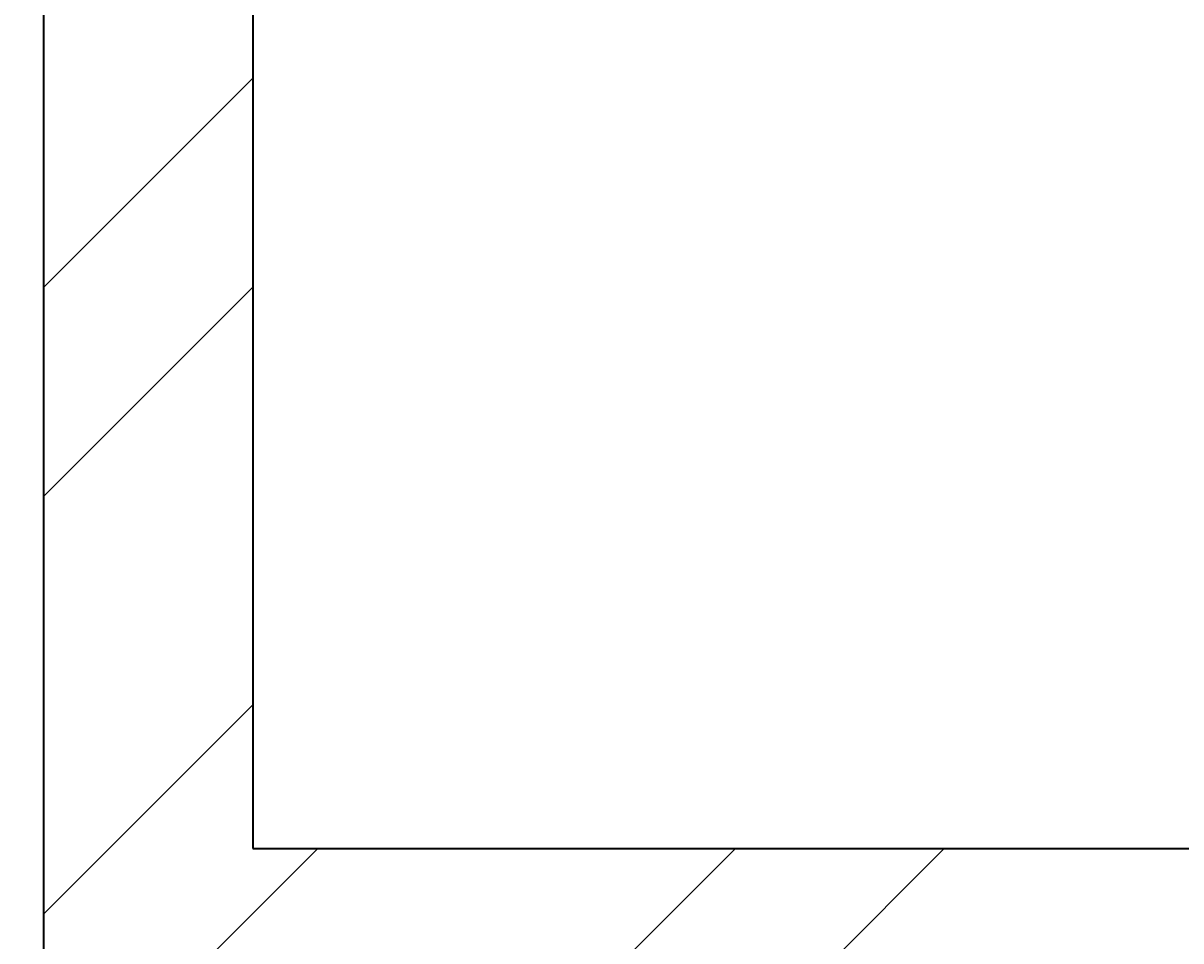
# Model space of a CAD drawing. Units: inches. Extents: x 1885 to 2748, y 783 to 2421.
# Tile 71 of 117: x 1992 to 2017, y 2073 to 2093. Entities that reach past the tile are written whole.
import ezdxf

# ---------------------------------------------------------------- set-up
doc = ezdxf.new("R2010")
doc.units = ezdxf.units.IN
doc.layers.add('A-ANNO-DIMS', color=2, linetype='Continuous', lineweight=18)
doc.layers.add('A-WALL', color=7, linetype='Continuous', lineweight=35)
doc.layers.add('A-WALL-PATT', color=85, linetype='Continuous', lineweight=13, true_color=0x58ba48)
doc.styles.get("Standard").update_dxf_attribs({"font": 'arial.ttf'})
doc.dimstyles.get("Standard").update_dxf_attribs({"dimtxt": 0.18, "dimasz": 0.18, "dimexe": 0.18, "dimexo": 0.0625, "dimgap": 0.09, "dimtad": 0, "dimtih": 1, "dimtoh": 1, "dimdec": 4, "dimzin": 0, "dimdsep": 46, "dimtxsty": 'Standard', "dimcen": 0.09, "dimadec": 0, "dimazin": 0, "dimtfac": 1, "dimtdec": 4, "dimtofl": 0, "dimtmove": 0, "dimatfit": 3, "dimfxl": 1, "dimtolj": 1, "dimtzin": 0, "dimarcsym": 0})

# ---------------------------------------------------------------- blocks, each defined once
blk = doc.blocks.new('*D48')
at = {"layer": 'A-ANNO-DIMS', "color": 0, "lineweight": -2, "transparency": 16777216}
for p, q in [((1980.711, 2348.006), (1902.844, 2348.006)), ((1903.024, 2347.826), (1903.024, 2114.937)), ((1903.024, 1881.686), (1903.024, 2114.574)), ((2016.711, 1881.506), (1902.844, 1881.506))]:
    blk.add_line(p, q, dxfattribs=at)
at = {"layer": 'A-ANNO-DIMS', "color": 0, "transparency": 16777216}
for points in [[(1902.994, 2347.826), (1903.054, 2347.826), (1903.024, 2348.006)], [(1902.994, 1881.686), (1903.054, 1881.686), (1903.024, 1881.506)]]:
    blk.add_solid(points, dxfattribs=at)
at = {"layer": 'Defpoints', "color": 0, "transparency": 16777216}
for p in [(1903.024, 2348.006), (1980.774, 2348.006), (2016.774, 1881.506)]:
    blk.add_point(p, dxfattribs=at)
at = {"layer": 'A-ANNO-DIMS', "color": 0, "transparency": 16777216, "insert": (1903.024, 2114.756), "char_height": 0.18, "attachment_point": 5}
blk.add_mtext('\\A1;466.5', dxfattribs=at)

msp = doc.modelspace()

# ---------------------------------------------------------------- hatches: boundary and pattern name
at = {"layer": 'A-WALL-PATT'}
h = msp.add_hatch(dxfattribs=at)
h.set_pattern_fill('ANSI32', color=256)
h.paths.add_polyline_path([(2007.772, 2318.006), (1980.774, 2318.006), (1980.774, 2281.215), (1985.274, 2281.215), (1985.274, 2313.506), (2007.772, 2313.506), (2007.772, 2315.756)])
h.paths.add_polyline_path([(2094.324, 2318.006), (2067.772, 2318.006), (2067.772, 2313.506), (2094.324, 2313.506), (2094.324, 2315.756)])
h.paths.add_polyline_path([(2131.367, 2315.756), (2131.367, 2318.006), (2131.189, 2318.006), (2112.609, 2318.006), (2112.609, 2313.506), (2117.274, 2313.506), (2117.274, 2255.201), (2121.774, 2255.201), (2121.774, 2313.506), (2131.367, 2313.506)])
h.paths.add_polyline_path([(2190.512, 2318.006), (2155.367, 2318.006), (2155.367, 2313.506), (2169.774, 2313.506), (2169.774, 2229.506), (2121.774, 2229.506), (2121.774, 2233.451), (2119.524, 2233.451), (2117.274, 2233.451), (2117.274, 2201.101), (2121.774, 2201.101), (2121.774, 2225.006), (2169.774, 2225.006), (2169.774, 2165.006), (2306.274, 2165.006), (2306.274, 2066.006), (2310.774, 2066.006), (2344.274, 2066.006), (2486.274, 2066.006), (2486.274, 1886.006), (2483.02, 1886.006), (2483.02, 1881.506), (2486.274, 1881.506), (2486.274, 1880.678), (2490.774, 1880.678), (2490.774, 2070.506), (2344.274, 2070.506), (2310.774, 2070.506), (2310.774, 2165.006), (2310.774, 2173.636), (2308.524, 2173.636), (2306.274, 2173.636), (2306.274, 2169.506), (2174.274, 2169.506), (2174.274, 2313.506), (2190.512, 2313.506), (2190.512, 2315.756)])
h.paths.add_polyline_path([(1985.274, 2221.215), (1980.774, 2221.215), (1980.774, 2165.006), (1992.774, 2165.006), (1992.774, 2141.927), (1997.274, 2141.927), (1997.274, 2165.006), (2117.274, 2165.006), (2117.274, 2163.126), (2121.774, 2163.126), (2121.774, 2172.734), (2119.524, 2172.734), (2117.274, 2172.734), (2117.274, 2169.506), (1985.274, 2169.506)])
h.paths.add_polyline_path([(1997.274, 2105.927), (1992.774, 2105.927), (1992.774, 2070.506), (2016.774, 2070.506), (2016.774, 2059.123), (2019.024, 2059.123), (2021.274, 2059.123), (2021.274, 2070.506), (2117.274, 2070.506), (2117.274, 2022.506), (2114.423, 2022.506), (2114.423, 2018.006), (2123.627, 2018.006), (2123.627, 2020.256), (2123.627, 2022.506), (2121.774, 2022.506), (2121.774, 2142.587), (2119.524, 2142.587), (2117.274, 2142.587), (2117.274, 2075.006), (1997.274, 2075.006)])
h.paths.add_polyline_path([(2092.029, 2020.256), (2092.029, 2022.506), (2021.274, 2022.506), (2021.274, 2035.123), (2016.774, 2035.123), (2016.774, 2018.006), (2016.774, 1978.784), (2021.274, 1978.784), (2021.274, 2018.006), (2092.029, 2018.006)])
h.paths.add_polyline_path([(2260.938, 2022.506), (2153.105, 2022.506), (2153.105, 2020.256), (2153.105, 2018.006), (2155.274, 2018.006), (2155.274, 1886.006), (2107.629, 1886.006), (2107.629, 1881.506), (2182.911, 1881.506), (2182.911, 1883.756), (2182.911, 1886.006), (2159.774, 1886.006), (2159.774, 2018.006), (2260.938, 2018.006), (2260.938, 2020.256)])
h.paths.add_polyline_path([(2047.629, 1883.756), (2047.629, 1886.006), (2021.274, 1886.006), (2021.274, 1918.784), (2019.024, 1918.784), (2016.774, 1918.784), (2016.774, 1881.506), (2047.629, 1881.506)])
h.paths.add_polyline_path([(2306.361, 1883.756), (2306.361, 1886.006), (2296.274, 1886.006), (2296.274, 1982.006), (2316.535, 1982.006), (2316.535, 1984.256), (2316.535, 1986.506), (2296.274, 1986.506), (2296.274, 2022.506), (2289.276, 2022.506), (2289.276, 2018.006), (2291.774, 2018.006), (2291.774, 1886.006), (2242.911, 1886.006), (2242.911, 1881.506), (2306.361, 1881.506)], flags=17)
h.paths.add_polyline_path([(1985.274, 1843.006), (2021.6, 1843.006), (2021.534, 1845.441), (2021.477, 1847.506), (1980.774, 1847.506), (1980.774, 1809.446), (1985.274, 1809.446)])
h.paths.add_polyline_path([(2131.482, 1845.256), (2131.482, 1847.506), (2081.534, 1847.506), (2081.534, 1843.006), (2117.274, 1843.006), (2117.274, 1784.147), (2119.524, 1784.147), (2121.774, 1784.147), (2121.774, 1843.006), (2131.482, 1843.006)])
h.paths.add_polyline_path([(2203.886, 1847.506), (2155.482, 1847.506), (2155.482, 1843.006), (2169.774, 1843.006), (2169.774, 1759.006), (2121.774, 1759.006), (2121.774, 1761.457), (2117.274, 1761.457), (2117.274, 1730.429), (2121.774, 1730.429), (2121.774, 1754.506), (2177.421, 1754.506), (2177.421, 1756.756), (2177.421, 1759.006), (2174.274, 1759.006), (2174.274, 1843.006), (2203.886, 1843.006)])
h.paths.add_polyline_path([(2335.554, 1845.256), (2335.554, 1847.506), (2239.886, 1847.506), (2239.886, 1843.006), (2306.274, 1843.006), (2306.274, 1759.006), (2199.486, 1759.006), (2199.486, 1754.506), (2310.774, 1754.506), (2310.774, 1843.006), (2335.554, 1843.006)])
h.paths.add_polyline_path([(2348.774, 2022.506), (2344.274, 2022.506), (2344.274, 1986.506), (2341.681, 1986.506), (2341.681, 1982.006), (2344.274, 1982.006), (2344.274, 1886.006), (2330.361, 1886.006), (2330.361, 1881.506), (2361.627, 1881.506), (2361.627, 1883.756), (2361.627, 1886.006), (2348.774, 1886.006)], flags=17)
h.paths.add_polyline_path([(2283.251, 2315.756), (2283.251, 2318.006), (2238.512, 2318.006), (2238.512, 2313.506), (2283.251, 2313.506)], flags=17)
h.paths.add_polyline_path([(2363.274, 2348.006), (2388.677, 2348.006), (2388.677, 2350.256), (2388.677, 2352.506), (2358.774, 2352.506), (2358.774, 2348.006), (2358.774, 2318.006), (2344.481, 2318.006), (2344.481, 2313.506), (2358.774, 2313.506), (2358.774, 2229.506), (2310.774, 2229.506), (2310.774, 2231.952), (2306.274, 2231.952), (2306.274, 2205.611), (2310.774, 2205.611), (2310.774, 2225.006), (2358.774, 2225.006), (2358.774, 2211.506), (2452.329, 2211.506), (2452.329, 2213.756), (2452.329, 2216.006), (2363.274, 2216.006), (2363.274, 2318.006)])
h.paths.add_polyline_path([(2310.774, 2313.506), (2320.481, 2313.506), (2320.481, 2315.756), (2320.481, 2318.006), (2302.728, 2318.006), (2302.728, 2313.506), (2306.274, 2313.506), (2306.274, 2251.076), (2310.774, 2251.076)], flags=17)
h.paths.add_polyline_path([(2490.774, 2352.506), (2486.274, 2352.506), (2448.677, 2352.506), (2448.677, 2348.006), (2486.274, 2348.006), (2486.274, 2318.006), (2486.274, 2216.006), (2481.78, 2216.006), (2481.78, 2211.506), (2486.274, 2211.506), (2486.274, 2165.006), (2493.289, 2165.006), (2493.289, 2167.256), (2493.289, 2169.506), (2490.774, 2169.506), (2490.774, 2313.506), (2494.429, 2313.506), (2494.429, 2318.006), (2490.774, 2318.006)])
h.paths.add_polyline_path([(2534.653, 2318.006), (2515.691, 2318.006), (2515.691, 2313.506), (2534.653, 2313.506), (2534.653, 2315.756)])
h.paths.add_polyline_path([(2618.274, 2318.006), (2594.653, 2318.006), (2594.653, 2313.506), (2613.774, 2313.506), (2613.774, 2281.706), (2618.274, 2281.706)])
h.paths.add_polyline_path([(2618.274, 2221.706), (2613.774, 2221.706), (2613.774, 2169.506), (2554.019, 2169.506), (2554.019, 2165.006), (2613.774, 2165.006), (2613.774, 2152.878), (2618.274, 2152.878)])
h.paths.add_polyline_path([(2618.274, 2128.878), (2616.024, 2128.878), (2613.774, 2128.878), (2613.774, 2117.006), (2529.774, 2117.006), (2529.774, 2165.006), (2532.848, 2165.006), (2532.848, 2169.506), (2522.867, 2169.506), (2522.867, 2165.006), (2525.274, 2165.006), (2525.274, 2117.006), (2525.274, 2112.506), (2525.274, 2108.576), (2529.774, 2108.576), (2529.774, 2112.506), (2613.774, 2112.506), (2613.774, 2080.19), (2618.274, 2080.19)])
h.paths.add_polyline_path([(2618.274, 2044.19), (2616.024, 2044.19), (2613.774, 2044.19), (2613.774, 2015.506), (2529.774, 2015.506), (2529.774, 2088.582), (2527.524, 2088.582), (2525.274, 2088.582), (2525.274, 2011.006), (2613.774, 2011.006), (2613.774, 1956.755), (2618.274, 1956.755)])
h.paths.add_polyline_path([(2618.274, 1881.506), (2618.274, 1896.755), (2613.774, 1896.755), (2613.774, 1881.506), (2613.774, 1847.506), (2592.715, 1847.506), (2592.715, 1843.006), (2613.774, 1843.006), (2613.774, 1765.006), (2613.774, 1760.506), (2609.621, 1760.506), (2609.621, 1756.006), (2613.774, 1756.006), (2613.774, 1660.006), (2608.544, 1660.006), (2608.544, 1655.506), (2613.774, 1655.506), (2613.774, 1508.158), (2618.274, 1508.158)])
h.paths.add_polyline_path([(2565.774, 1843.006), (2568.997, 1843.006), (2568.997, 1847.506), (2490.774, 1847.506), (2490.774, 1849.7), (2488.524, 1849.7), (2486.274, 1849.7), (2486.274, 1847.506), (2477.274, 1847.506), (2477.274, 1838.506), (2477.274, 1821.493), (2486.274, 1821.493), (2486.274, 1838.506), (2561.274, 1838.506), (2561.274, 1765.006), (2486.274, 1765.006), (2486.274, 1786.157), (2477.274, 1786.157), (2477.274, 1765.006), (2477.274, 1756.006), (2486.274, 1756.006), (2565.774, 1756.006), (2585.621, 1756.006), (2585.621, 1758.256), (2585.621, 1760.506), (2565.774, 1760.506), (2565.774, 1765.006)])
h.paths.add_polyline_path([(2486.274, 1651.006), (2561.274, 1651.006), (2561.274, 1567.006), (2486.274, 1567.006), (2486.274, 1591.321), (2477.274, 1591.321), (2477.274, 1567.006), (2477.274, 1558.006), (2477.274, 1555.439), (2481.774, 1555.439), (2481.774, 1558.006), (2568.653, 1558.006), (2568.653, 1560.256), (2568.653, 1562.506), (2565.774, 1562.506), (2565.774, 1655.506), (2584.544, 1655.506), (2584.544, 1657.756), (2584.544, 1660.006), (2565.774, 1660.006), (2486.274, 1660.006), (2477.274, 1660.006), (2477.274, 1651.006), (2477.274, 1632.989), (2486.274, 1632.989)])
h.paths.add_polyline_path([(2449.967, 1883.756), (2449.967, 1886.006), (2421.627, 1886.006), (2421.627, 1881.506), (2449.967, 1881.506)], flags=17)
h.paths.add_polyline_path([(2447.274, 1847.506), (2395.554, 1847.506), (2395.554, 1843.006), (2442.774, 1843.006), (2442.774, 1809.27), (2447.274, 1809.27)])
h.paths.add_polyline_path([(1985.274, 1749.446), (1980.774, 1749.446), (1980.774, 1694.504), (1985.274, 1694.504), (1985.274, 1694.506), (1986.897, 1694.506), (1986.897, 1697.78), (1986.897, 1699.006), (1985.274, 1699.006)])
h.paths.add_polyline_path([(2152.774, 1699.006), (2121.774, 1699.006), (2121.774, 1703.668), (2119.524, 1703.668), (2117.274, 1703.668), (2117.274, 1699.006), (2009.219, 1699.006), (2009.219, 1694.506), (2148.274, 1694.506), (2148.274, 1692.631), (2152.774, 1692.631)])
h.paths.add_polyline_path([(2016.274, 1694.506), (2011.774, 1694.506), (2011.774, 1558.006), (2040.806, 1558.006), (2040.806, 1560.256), (2040.806, 1562.506), (2016.274, 1562.506)])
h.paths.add_polyline_path([(2152.774, 1663.017), (2150.524, 1663.017), (2148.274, 1663.017), (2148.274, 1562.506), (2100.806, 1562.506), (2100.806, 1558.006), (2165.119, 1558.006), (2165.119, 1560.256), (2165.119, 1562.506), (2152.774, 1562.506), (2152.774, 1610.506), (2224.774, 1610.506), (2224.774, 1607.99), (2229.274, 1607.99), (2229.274, 1615.006), (2152.774, 1615.006)])
h.paths.add_polyline_path([(2238.613, 1560.256), (2238.613, 1562.506), (2229.274, 1562.506), (2229.274, 1588.756), (2227.024, 1588.763), (2224.774, 1588.771), (2224.774, 1562.506), (2189.119, 1562.506), (2189.119, 1558.006), (2238.613, 1558.006)])
h.paths.add_polyline_path([(2336.024, 1560.256), (2336.024, 1562.506), (2310.774, 1562.506), (2310.774, 1656.347), (2308.524, 1656.347), (2306.274, 1656.347), (2306.274, 1562.506), (2286.613, 1562.506), (2286.613, 1558.006), (2336.024, 1558.006)])
h.paths.add_polyline_path([(2447.274, 1690.968), (2445.024, 1690.968), (2442.774, 1690.968), (2442.774, 1687.006), (2306.274, 1687.006), (2306.274, 1680.75), (2310.774, 1680.75), (2310.774, 1682.506), (2442.774, 1682.506), (2442.774, 1562.506), (2396.024, 1562.506), (2396.024, 1558.006), (2447.274, 1558.006)])
h.paths.add_polyline_path([(2447.274, 1749.27), (2445.024, 1749.27), (2442.774, 1749.27), (2442.774, 1717.232), (2447.274, 1717.232)])
h.paths.add_polyline_path([(2044.674, 1521.756), (2044.674, 1524.006), (2007.274, 1524.006), (2007.274, 1503.49), (2009.524, 1503.49), (2011.774, 1503.49), (2011.774, 1519.506), (2044.674, 1519.506)])
h.paths.add_polyline_path([(2177.969, 1521.756), (2177.969, 1524.006), (2104.674, 1524.006), (2104.674, 1519.506), (2145.774, 1519.506), (2145.774, 1387.506), (2143.37, 1387.506), (2143.37, 1383.006), (2251.585, 1383.006), (2251.585, 1385.256), (2251.585, 1387.506), (2150.274, 1387.506), (2150.274, 1519.506), (2177.969, 1519.506)])
h.paths.add_polyline_path([(2298.704, 1524.006), (2237.969, 1524.006), (2237.969, 1519.506), (2282.274, 1519.506), (2282.274, 1387.506), (2279.683, 1387.506), (2279.683, 1383.006), (2286.774, 1383.006), (2286.774, 1419.006), (2312.451, 1419.006), (2312.451, 1421.256), (2312.451, 1423.506), (2286.774, 1423.506), (2286.774, 1519.506), (2298.704, 1519.506), (2298.704, 1521.722)], flags=17)
h.paths.add_polyline_path([(2361.897, 1521.756), (2361.897, 1524.006), (2322.704, 1524.006), (2322.704, 1519.506), (2334.774, 1519.506), (2334.774, 1423.506), (2331.93, 1423.506), (2331.93, 1419.006), (2334.774, 1419.006), (2334.774, 1387.506), (2334.774, 1383.228), (2339.274, 1383.228), (2339.274, 1387.506), (2339.274, 1519.506), (2361.897, 1519.506)], flags=17)
h.paths.add_polyline_path([(2447.274, 1521.756), (2447.274, 1524.006), (2421.897, 1524.006), (2421.897, 1519.506), (2447.274, 1519.506)], flags=17)
h.paths.add_polyline_path([(2481.774, 1529.6), (2479.524, 1529.6), (2477.274, 1529.6), (2477.274, 1524.006), (2474.489, 1524.006), (2474.489, 1519.506), (2477.274, 1519.506), (2477.274, 1334.506), (2296.774, 1334.506), (2296.774, 1240.506), (2160.274, 1240.506), (2160.274, 1180.506), (2112.274, 1180.506), (2112.274, 1207.692), (2110.024, 1207.692), (2107.774, 1207.692), (2107.774, 1171.609), (2112.274, 1171.609), (2112.274, 1176.006), (2160.274, 1176.006), (2160.274, 1092.006), (2144.221, 1092.006), (2144.221, 1087.506), (2189.497, 1087.506), (2189.497, 1089.756), (2189.497, 1092.006), (2164.774, 1092.006), (2164.774, 1236.006), (2296.774, 1236.006), (2296.774, 1231.912), (2301.274, 1231.912), (2301.274, 1330.006), (2481.774, 1330.006), (2481.774, 1387.506)])
h.paths.add_polyline_path([(2618.274, 1448.158), (2613.774, 1448.158), (2613.774, 1382.506), (2529.774, 1382.506), (2525.274, 1382.506), (2525.274, 1307.062), (2529.774, 1307.062), (2529.774, 1378.006), (2613.774, 1378.006), (2613.774, 1354.988), (2618.274, 1354.988)])
h.paths.add_polyline_path([(2618.274, 1318.988), (2613.774, 1318.988), (2613.774, 1281.006), (2529.774, 1281.006), (2529.774, 1283.786), (2527.524, 1283.786), (2525.274, 1283.786), (2525.274, 1228.506), (2516.794, 1228.506), (2516.794, 1224.006), (2533.484, 1224.006), (2533.484, 1226.256), (2533.484, 1228.506), (2529.774, 1228.506), (2529.774, 1276.506), (2613.774, 1276.506), (2613.774, 1266.02), (2618.274, 1266.02)])
h.paths.add_polyline_path([(2618.274, 1134.964), (2613.774, 1134.964), (2613.774, 1092.006), (2594.545, 1092.006), (2594.545, 1087.506), (2618.274, 1087.506)])
h.paths.add_polyline_path([(2534.545, 1092.006), (2509.765, 1092.006), (2509.765, 1087.506), (2534.545, 1087.506), (2534.545, 1089.756)])
h.paths.add_polyline_path([(2481.274, 1224.006), (2484.117, 1224.006), (2484.117, 1226.256), (2484.117, 1228.506), (2476.774, 1228.506), (2476.774, 1198.506), (2471.61, 1198.506), (2471.61, 1194.006), (2476.774, 1194.006), (2476.774, 1062.006), (2436.894, 1062.006), (2436.894, 1057.506), (2476.774, 1057.506), (2481.274, 1057.506), (2481.274, 1062.006), (2481.274, 1087.506), (2485.354, 1087.506), (2485.354, 1089.756), (2485.354, 1092.006), (2481.274, 1092.006), (2481.274, 1117.506)])
h.paths.add_polyline_path([(2439.898, 1198.506), (2349.274, 1198.506), (2349.274, 1194.006), (2349.274, 1180.506), (2301.274, 1180.506), (2301.274, 1201.896), (2299.024, 1201.896), (2296.774, 1201.896), (2296.774, 1172.335), (2299.024, 1172.335), (2301.274, 1172.335), (2301.274, 1176.006), (2349.274, 1176.006), (2349.274, 1092.006), (2334.452, 1092.006), (2334.452, 1087.506), (2349.274, 1087.506), (2349.274, 1057.506), (2353.774, 1057.506), (2376.894, 1057.506), (2376.894, 1059.756), (2376.894, 1062.006), (2353.774, 1062.006), (2353.774, 1087.506), (2353.774, 1180.506), (2353.774, 1194.006), (2439.898, 1194.006), (2439.898, 1196.256)])
h.paths.add_polyline_path([(2270.596, 1089.756), (2270.596, 1092.006), (2249.497, 1092.006), (2249.497, 1087.506), (2270.596, 1087.506)], flags=17)
h.paths.add_polyline_path([(2310.452, 1092.006), (2301.274, 1092.006), (2301.274, 1153.292), (2296.774, 1153.292), (2296.774, 1092.006), (2293.786, 1092.006), (2293.786, 1087.506), (2310.452, 1087.506), (2310.452, 1089.756)], flags=17)
h.paths.add_polyline_path([(2112.274, 1150.328), (2110.024, 1150.328), (2107.774, 1150.328), (2107.774, 1092.006), (2104.465, 1092.006), (2104.465, 1087.506), (2120.221, 1087.506), (2120.221, 1089.756), (2120.221, 1092.006), (2112.274, 1092.006)])
h.paths.add_polyline_path([(2082.172, 1092.006), (2058.144, 1092.006), (2058.144, 1087.506), (2082.172, 1087.506), (2082.172, 1089.756)])
h.paths.add_polyline_path([(1975.774, 1145.638), (1971.274, 1145.638), (1971.274, 1087.506), (1980.774, 1087.506), (1998.144, 1087.506), (1998.144, 1089.756), (1998.144, 1092.006), (1985.274, 1092.006), (1975.774, 1092.006)])
h.paths.add_polyline_path([(2112.274, 1244.385), (2110.024, 1244.385), (2107.774, 1244.385), (2107.774, 1240.506), (1992.274, 1240.506), (1992.274, 1271.008), (1987.774, 1271.008), (1987.774, 1240.506), (1980.774, 1240.506), (1975.774, 1240.506), (1971.274, 1240.506), (1971.274, 1205.638), (1975.774, 1205.638), (1975.774, 1236.006), (2107.774, 1236.006), (2107.774, 1233.444), (2112.274, 1233.444), (2112.274, 1236.006)])
h.paths.add_polyline_path([(2112.274, 1383.006), (2114.783, 1383.006), (2114.783, 1385.256), (2114.783, 1387.506), (2102.476, 1387.506), (2102.476, 1383.006), (2107.774, 1383.006), (2107.774, 1335.006), (2011.774, 1335.006), (2011.774, 1349.939), (2007.274, 1349.939), (2007.274, 1335.006), (1987.774, 1335.006), (1987.774, 1330.506), (1987.774, 1307.008), (1992.274, 1307.008), (1992.274, 1330.506), (2007.274, 1330.506), (2107.774, 1330.506), (2107.774, 1264.711), (2112.274, 1264.711)])
h.paths.add_polyline_path([(2077.857, 1387.506), (2011.774, 1387.506), (2011.774, 1390.036), (2009.524, 1390.036), (2007.274, 1390.036), (2007.274, 1373.939), (2011.774, 1373.939), (2011.774, 1383.006), (2077.857, 1383.006)])
h.paths.add_polyline_path([(2011.774, 1443.49), (2007.274, 1443.49), (2007.274, 1410.248), (2011.774, 1410.248)])

# ---------------------------------------------------------------- linework, layer by layer
at = {"layer": 'A-WALL'}
for p, q in [((1992.774, 2105.927), (1992.774, 2070.506)), ((1997.274, 2105.927), (1997.274, 2075.006)), ((1997.274, 2075.006), (2117.274, 2075.006))]:
    msp.add_line(p, q, dxfattribs=at)

# ---------------------------------------------------------------- dimensions: what is measured, and where the dimension line sits
at = {"layer": 'A-ANNO-DIMS'}
dim = msp.add_linear_dim(base=(1903.024, 2348.006), p1=(2016.774, 1881.506), p2=(1980.774, 2348.006), angle=90, dimstyle='Standard', override={"dimdec": 1, "dimlfac": 1, "dimrnd": 0, "dimzin": 0, "dimdsep": 46, "dimlunit": 2}, dxfattribs=at)
dim.commit()
dim.dimension.update_dxf_attribs({"geometry": '*D48', "text_midpoint": (1903.024, 2114.756)})

doc.saveas('drawing.dxf')
